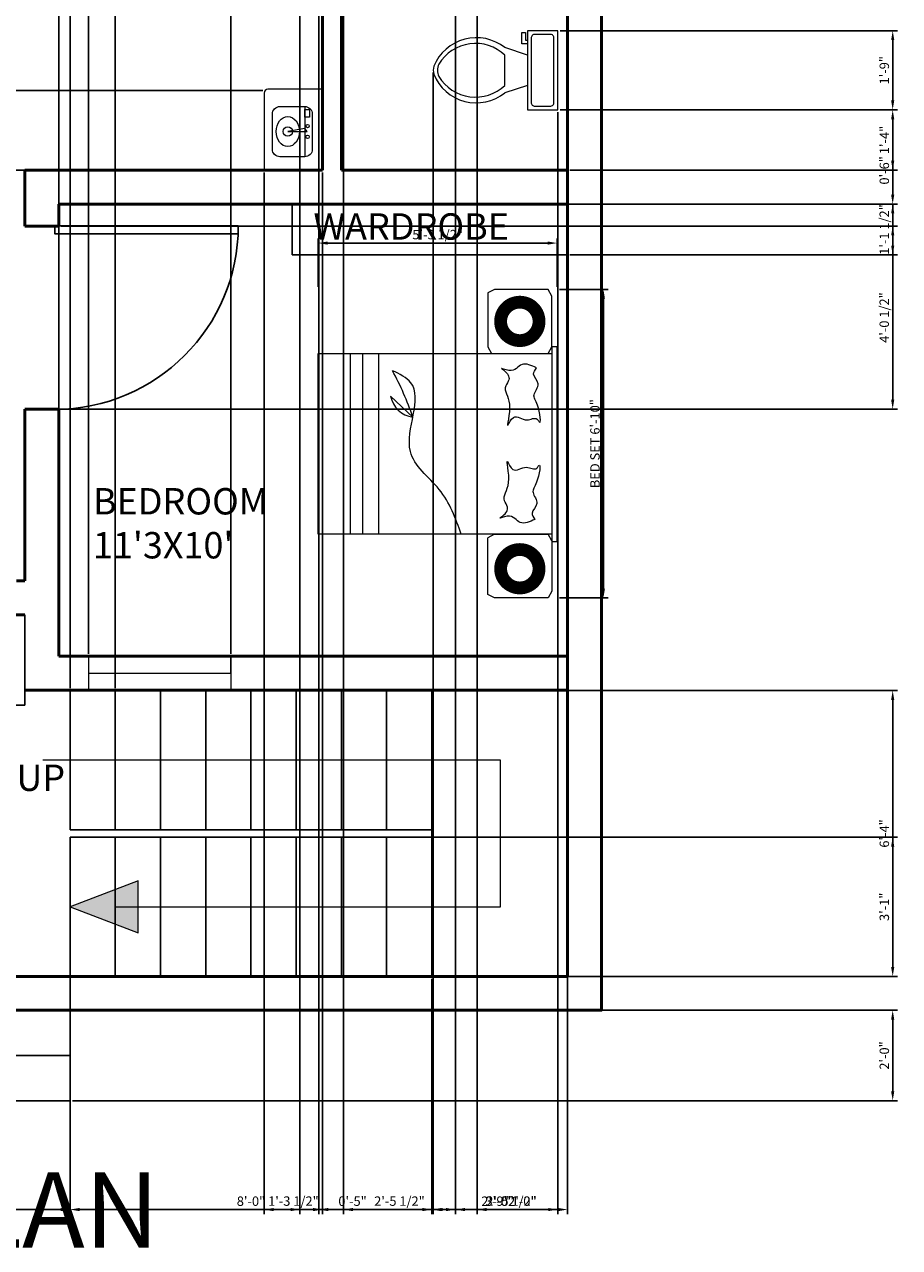
# Model space of a CAD drawing. Units: inches. Extents: x 1854 to 2268, y 1958 to 2535.
# Tile 2 of 4: x 2035 to 2268, y 1958 to 2283. Entities that reach past the tile are written whole.
import ezdxf

# ---------------------------------------------------------------- set-up
doc = ezdxf.new("R2010")
doc.units = ezdxf.units.IN
for name, color, linetype, lineweight in [('A-ANNO-DIMS', 2, 'Continuous', 18), ('A-ANNO-SYMB', 7, 'Continuous', 18), ('A-ANNO-TEXT', 7, 'Continuous', 25), ('A-AREA-IDEN', 7, 'Continuous', 25), ('A-DOOR', 3, 'Continuous', 25), ('A-FLOR-CASE', 30, 'Continuous', 25), ('A-FLOR-FIXT', 9, 'Continuous', 18), ('A-FLOR-STRS', 7, 'Continuous', 25), ('A-FURN', 8, 'Continuous', 18), ('A-GLAZ', 4, 'Continuous', 18), ('A-WALL', 7, 'Continuous', 50)]:
    doc.layers.add(name, color=color, linetype=linetype, lineweight=lineweight)
doc.styles.get("Standard").update_dxf_attribs({"font": 'arial.ttf'})
doc.dimstyles.new('ISO-25', dxfattribs={"dimtxt": 2.5, "dimasz": 2.5, "dimexe": 1.25, "dimexo": 0.625, "dimtad": 1, "dimdec": 0, "dimlunit": 3, "dimtxsty": 'Standard', "dimcen": 2.5, "dimadec": 0, "dimazin": 0, "dimtfac": 1, "dimtdec": 0, "dimtmove": 0, "dimatfit": 3, "dimfxl": 1, "dimarcsym": 0})

# ---------------------------------------------------------------- blocks, each defined once
blk = doc.blocks.new('bed 123')
for p, q in [((-25.76, 31), (25.94, 31)), ((25.94, 32.39), (-25.74, 32.39)), ((-25.74, 32.39), (-25.74, 31)), ((25.76, 31), (24, 30.06)), ((24, 15.76), (24, 30.06)), ((25.76, 31), (39.15, 31)), ((25.94, 31), (25.94, 32.39)), ((39.15, 31), (40.91, 30.06)), ((40.91, 30.06), (40.91, 15.76)), ((24, 15.76), (24.94, 14)), ((39.97, 14), (24.94, 14)), ((40.91, 15.76), (39.97, 14)), ((24, 2.1), (24, -31)), ((-7.1, -5.89), (-12.68, -11.78)), ((-24, -15.04), (24, -15.04)), ((-24, -19.27), (24, -19.27)), ((-24, -22.54), (24, -22.54)), ((-10.17, -31), (-7.61, -31.01))]:
    blk.add_line(p, q)
for points in [[(-25.76, 31), (-39.24, 31), (-41, 30.06), (-41, 15.76), (-40.06, 14), (-25.76, 14), (-24, 14.94), (-24, 30.06)], [(-24, 31), (24, 31), (24, -31), (-24, -31)]]:
    blk.add_lwpolyline(points, close=True)
at = {"const_width": 3.4}
for points in [[(-37.6, 22.5, 1), (-27.4, 22.5, 1)], [(28.06, 22.5, 1), (38.25, 22.5, 1)]]:
    blk.add_lwpolyline(points, format="xyb", close=True, dxfattribs=at)
for centre, radius, start, end in [((18.98, -82.09), 80.54, 108.8924, 118.4699), ((-13.83, -5.1), 6.78, 279.7804, 353.3519)]:
    blk.add_arc(centre, radius, start, end)
for points, knots in [([(-20.15, 26.95), (-19.6, 26.55), (-18.19, 25.51), (-15.93, 28.42), (-12.93, 25.48), (-10.53, 27.62), (-4.31, 28.37), (-7.37, 26.8), (-5.38, 23.99), (-8.44, 20.96), (-2.62, 18.36), (-11.44, 21), (-14.41, 17.7), (-17.27, 20.15), (-18.97, 19.07), (-20.5, 16.88), (-18.47, 20.9), (-22.11, 22.82), (-20.81, 25.56), (-20.15, 26.95)], [0, 0, 0, 0, 1.83091, 4.653214, 7.743318, 10.66504, 15.119925, 15.953636, 18.69724, 22.356007, 24.774329, 30.270914, 35.21341, 37.060797, 39.714351, 40.728626, 42.795822, 46.625816, 50.594847, 50.594847, 50.594847, 50.594847]), ([(20.06, 26.52), (19.49, 26.12), (18.07, 25.12), (15.87, 28.07), (12.81, 25.2), (10.45, 27.4), (4.25, 28.28), (7.28, 26.65), (5.23, 23.88), (8.23, 20.78), (2.35, 18.31), (11.22, 20.76), (14.12, 17.4), (17.03, 19.78), (18.71, 18.67), (20.2, 16.44), (18.25, 20.5), (21.92, 22.34), (20.69, 25.11), (20.06, 26.52)], [0, 0, 0, 0, 1.83091, 4.653214, 7.743318, 10.66504, 15.119925, 15.953636, 18.69724, 22.356007, 24.774329, 30.270914, 35.21341, 37.060797, 39.714351, 40.728626, 42.795822, 46.625816, 50.594847, 50.594847, 50.594847, 50.594847]), ([(24, 6.96), (19.8, 5.46), (11.61, 2.51), (2.01, -11.3), (-14.71, -1.57), (-18.5, -9.41), (-19.41, -11.29)], [0, 0, 0, 0, 13.291621, 25.945947, 44.21489, 49.956985, 49.956985, 49.956985, 49.956985])]:
    blk.add_open_spline(points, degree=3, knots=knots)
blk = doc.blocks.new('*U10')
for p, q in [((9.5, -6), (9.5, -2)), ((-10, -8.5), (-8, -8.5)), ((-10, -9.5), (-10, -8.5)), ((-7, -9.5), (-10, -9.5)), ((-8, -8.5), (-8, -8)), ((-7, -8), (-7, -9.5)), ((-4, -8), (-6, -14)), ((4, -8), (6, -14)), ((4, -14), (-4, -14))]:
    blk.add_line(p, q)
blk.add_lwpolyline([(10.5, -8), (10.5, 0), (-10.5, 0), (-10.5, -8)], close=True)
for points in [[(-9.5, -2), (-9.5, -6)], [(8.5, -1), (-8.5, -1)], [(-8.5, -7), (8.5, -7)]]:
    blk.add_lwpolyline(points)
for centre, radius, start, end in [((-8.62, -1.88), 0.884, 81.8699, 188.1301), ((8.62, -1.88), 0.884, 351.8699, 98.1301), ((-8.62, -6.12), 0.884, 171.8699, 278.1301), ((8.62, -6.12), 0.884, 261.8699, 8.1301), ((3.52, -21.58), 12.17, 141.4691, 247.9714), ((4.2, -21.82), 11.33, 136.3677, 238.9468), ((-3.52, -21.58), 12.17, 292.0284, 38.5307), ((-4.2, -21.82), 11.33, 301.053, 43.6321), ((0, -27.88), 4, 245.7318, 294.2682), ((0, -29), 4, 254.8605, 285.1395)]:
    blk.add_arc(centre, radius, start, end)
blk = doc.blocks.new('*U13')
for p, q in [((-40, 0), (-40, 6)), ((0, 0), (0, 6))]:
    blk.add_line(p, q)
blk.add_lwpolyline([(0, 0), (0, -40), (-1.75, -40), (-1.75, 0)], close=True)
blk.add_arc((0, 0), 40, 180, 270)
blk = doc.blocks.new('*D23')
at = {"layer": 'A-ANNO-DIMS', "color": 0, "lineweight": -2, "transparency": 16777216}
for p, q in [((2177.29, 2212.2), (2190.2, 2212.2)), ((2188.95, 2209.7), (2188.95, 2132.79)), ((2177.29, 2130.29), (2190.2, 2130.29))]:
    blk.add_line(p, q, dxfattribs=at)
at = {"layer": 'A-ANNO-DIMS', "color": 0, "transparency": 16777216}
for points in [[(2188.53, 2209.7), (2189.36, 2209.7), (2188.95, 2212.2)], [(2188.53, 2132.79), (2189.36, 2132.79), (2188.95, 2130.29)]]:
    blk.add_solid(points, dxfattribs=at)
at = {"layer": 'Defpoints', "color": 0, "transparency": 16777216}
for p in [(2176.66, 2212.2), (2176.66, 2130.29), (2188.95, 2130.29)]:
    blk.add_point(p, dxfattribs=at)
at = {"layer": 'A-ANNO-DIMS', "color": 0, "transparency": 16777216, "insert": (2187.03, 2171.25), "char_height": 2.5, "attachment_point": 5, "rotation": 90}
blk.add_mtext('BED SET 6\'-10"', dxfattribs=at)
blk = doc.blocks.new('*D24')
at = {"layer": 'A-ANNO-DIMS', "color": 0, "lineweight": -2, "transparency": 16777216}
for p, q in [((2113.26, 2212.83), (2113.26, 2225.74)), ((2115.76, 2224.49), (2174.16, 2224.49)), ((2176.66, 2212.83), (2176.66, 2225.74))]:
    blk.add_line(p, q, dxfattribs=at)
at = {"layer": 'A-ANNO-DIMS', "color": 0, "transparency": 16777216}
for points in [[(2115.76, 2224.91), (2115.76, 2224.07), (2113.26, 2224.49)], [(2174.16, 2224.91), (2174.16, 2224.07), (2176.66, 2224.49)]]:
    blk.add_solid(points, dxfattribs=at)
at = {"layer": 'Defpoints', "color": 0, "transparency": 16777216}
for p in [(2176.66, 2224.49), (2113.26, 2212.2), (2176.66, 2212.2)]:
    blk.add_point(p, dxfattribs=at)
at = {"layer": 'A-ANNO-DIMS', "color": 0, "transparency": 16777216, "insert": (2144.96, 2226.41), "char_height": 2.5, "attachment_point": 5}
blk.add_mtext('5\'-3 1/2"', dxfattribs=at)
blk = doc.blocks.new('*D36')
at = {"layer": 'A-ANNO-DIMS', "color": 0, "lineweight": -2, "transparency": 16777216}
for p, q in [((2119.96, 2378.21), (2119.96, 1966.69)), ((2149.7, 2378.21), (2149.7, 1966.69)), ((2122.46, 1967.94), (2147.2, 1967.94))]:
    blk.add_line(p, q, dxfattribs=at)
at = {"layer": 'A-ANNO-DIMS', "color": 0, "transparency": 16777216}
for points in [[(2122.46, 1968.36), (2122.46, 1967.52), (2119.96, 1967.94)], [(2147.2, 1968.36), (2147.2, 1967.52), (2149.7, 1967.94)]]:
    blk.add_solid(points, dxfattribs=at)
at = {"layer": 'Defpoints', "color": 0, "transparency": 16777216}
for p in [(2119.96, 2378.84), (2149.7, 2378.84), (2149.7, 1967.94)]:
    blk.add_point(p, dxfattribs=at)
at = {"layer": 'A-ANNO-DIMS', "color": 0, "transparency": 16777216, "insert": (2134.83, 1969.86), "char_height": 2.5, "attachment_point": 5}
blk.add_mtext('2\'-5 1/2"', dxfattribs=at)
blk = doc.blocks.new('*D38')
at = {"layer": 'A-ANNO-DIMS', "color": 0, "lineweight": -2, "transparency": 16777216}
for p, q in [((2045.06, 2229.02), (2266.96, 2229.02)), ((2265.71, 2226.52), (2265.71, 2182.92)), ((2045.06, 2180.42), (2266.96, 2180.42))]:
    blk.add_line(p, q, dxfattribs=at)
at = {"layer": 'A-ANNO-DIMS', "color": 0, "transparency": 16777216}
for points in [[(2265.29, 2226.52), (2266.13, 2226.52), (2265.71, 2229.02)], [(2265.29, 2182.92), (2266.13, 2182.92), (2265.71, 2180.42)]]:
    blk.add_solid(points, dxfattribs=at)
at = {"layer": 'Defpoints', "color": 0, "transparency": 16777216}
for p in [(2044.43, 2229.02), (2044.43, 2180.42), (2265.71, 2180.42)]:
    blk.add_point(p, dxfattribs=at)
at = {"layer": 'A-ANNO-DIMS', "color": 0, "transparency": 16777216, "insert": (2263.79, 2204.72), "char_height": 2.5, "attachment_point": 5, "rotation": 90}
blk.add_mtext('4\'-0 1/2"', dxfattribs=at)
blk = doc.blocks.new('*D43')
at = {"layer": 'A-ANNO-DIMS', "color": 0, "lineweight": -2, "transparency": 16777216}
for p, q in [((2052.36, 2115.46), (2052.36, 2530.99)), ((2054.86, 2529.74), (2087.6, 2529.74)), ((2090.1, 2115.46), (2090.1, 2530.99))]:
    blk.add_line(p, q, dxfattribs=at)
at = {"layer": 'A-ANNO-DIMS', "color": 0, "transparency": 16777216}
for points in [[(2054.86, 2530.16), (2054.86, 2529.32), (2052.36, 2529.74)], [(2087.6, 2530.16), (2087.6, 2529.32), (2090.1, 2529.74)]]:
    blk.add_solid(points, dxfattribs=at)
at = {"layer": 'Defpoints', "color": 0, "transparency": 16777216}
for p in [(2090.1, 2529.74), (2052.36, 2114.84), (2090.1, 2114.84)]:
    blk.add_point(p, dxfattribs=at)
at = {"layer": 'A-ANNO-DIMS', "color": 0, "transparency": 16777216, "insert": (2071.23, 2531.66), "char_height": 2.5, "attachment_point": 5}
blk.add_mtext('3\'-1 1/2"', dxfattribs=at)
blk = doc.blocks.new('*D45')
at = {"layer": 'A-ANNO-DIMS', "color": 0, "lineweight": -2, "transparency": 16777216}
for p, q in [((1906.99, 2001.07), (1906.99, 1966.69)), ((2047.43, 1996.21), (2047.43, 1966.69)), ((1909.49, 1967.94), (2044.93, 1967.94))]:
    blk.add_line(p, q, dxfattribs=at)
at = {"layer": 'A-ANNO-DIMS', "color": 0, "transparency": 16777216}
for points in [[(1909.49, 1968.36), (1909.49, 1967.52), (1906.99, 1967.94)], [(2044.93, 1968.36), (2044.93, 1967.52), (2047.43, 1967.94)]]:
    blk.add_solid(points, dxfattribs=at)
at = {"layer": 'Defpoints', "color": 0, "transparency": 16777216}
for p in [(1906.99, 2001.7), (2047.43, 1996.84), (2047.43, 1967.94)]:
    blk.add_point(p, dxfattribs=at)
at = {"layer": 'A-ANNO-DIMS', "color": 0, "transparency": 16777216, "insert": (1977.21, 1969.86), "char_height": 2.5, "attachment_point": 5}
blk.add_mtext('11\'-8 1/2"', dxfattribs=at)
blk = doc.blocks.new('*D46')
at = {"layer": 'A-ANNO-DIMS', "color": 0, "lineweight": -2, "transparency": 16777216}
for p, q in [((2048.06, 2020.84), (2266.96, 2020.84)), ((2265.71, 2018.34), (2265.71, 1999.34)), ((2048.06, 1996.84), (2266.96, 1996.84))]:
    blk.add_line(p, q, dxfattribs=at)
at = {"layer": 'A-ANNO-DIMS', "color": 0, "transparency": 16777216}
for points in [[(2265.29, 2018.34), (2266.13, 2018.34), (2265.71, 2020.84)], [(2265.29, 1999.34), (2266.13, 1999.34), (2265.71, 1996.84)]]:
    blk.add_solid(points, dxfattribs=at)
at = {"layer": 'Defpoints', "color": 0, "transparency": 16777216}
for p in [(2047.43, 2020.84), (2047.43, 1996.84), (2265.71, 1996.84)]:
    blk.add_point(p, dxfattribs=at)
at = {"layer": 'A-ANNO-DIMS', "color": 0, "transparency": 16777216, "insert": (2263.81, 2008.84), "char_height": 2.5, "attachment_point": 5, "rotation": 90}
blk.add_mtext('2\'-0"', dxfattribs=at)
blk = doc.blocks.new('*D47')
at = {"layer": 'A-ANNO-DIMS', "color": 0, "lineweight": -2, "transparency": 16777216}
for p, q in [((2143.43, 2029.22), (2143.43, 1966.69)), ((2047.43, 2020.21), (2047.43, 1966.69)), ((2049.93, 1967.94), (2140.93, 1967.94))]:
    blk.add_line(p, q, dxfattribs=at)
at = {"layer": 'A-ANNO-DIMS', "color": 0, "transparency": 16777216}
for points in [[(2049.93, 1968.36), (2049.93, 1967.52), (2047.43, 1967.94)], [(2140.93, 1968.36), (2140.93, 1967.52), (2143.43, 1967.94)]]:
    blk.add_solid(points, dxfattribs=at)
at = {"layer": 'Defpoints', "color": 0, "transparency": 16777216}
for p in [(2143.43, 2029.84), (2047.43, 2020.84), (2143.43, 1967.94)]:
    blk.add_point(p, dxfattribs=at)
at = {"layer": 'A-ANNO-DIMS', "color": 0, "transparency": 16777216, "insert": (2095.43, 1969.84), "char_height": 2.5, "attachment_point": 5}
blk.add_mtext('8\'-0"', dxfattribs=at)
blk = doc.blocks.new('*D48')
at = {"layer": 'A-ANNO-DIMS', "color": 0, "lineweight": -2, "transparency": 16777216}
for p, q in [((2144.06, 2105.7), (2266.96, 2105.7)), ((2265.71, 2032.34), (2265.71, 2103.2)), ((2144.06, 2029.84), (2266.96, 2029.84))]:
    blk.add_line(p, q, dxfattribs=at)
at = {"layer": 'A-ANNO-DIMS', "color": 0, "transparency": 16777216}
for points in [[(2265.29, 2103.2), (2266.13, 2103.2), (2265.71, 2105.7)], [(2265.29, 2032.34), (2266.13, 2032.34), (2265.71, 2029.84)]]:
    blk.add_solid(points, dxfattribs=at)
at = {"layer": 'Defpoints', "color": 0, "transparency": 16777216}
for p in [(2143.43, 2105.7), (2265.71, 2105.7), (2143.43, 2029.84)]:
    blk.add_point(p, dxfattribs=at)
at = {"layer": 'A-ANNO-DIMS', "color": 0, "transparency": 16777216, "insert": (2263.81, 2067.77), "char_height": 2.5, "attachment_point": 5, "rotation": 90}
blk.add_mtext('6\'-4"', dxfattribs=at)
blk = doc.blocks.new('*D52')
at = {"layer": 'A-ANNO-DIMS', "color": 0, "lineweight": -2, "transparency": 16777216}
for p, q in [((2149.7, 2378.21), (2149.7, 1966.69)), ((2179.43, 2378.21), (2179.43, 1966.69)), ((2152.2, 1967.94), (2176.93, 1967.94))]:
    blk.add_line(p, q, dxfattribs=at)
at = {"layer": 'A-ANNO-DIMS', "color": 0, "transparency": 16777216}
for points in [[(2152.2, 1968.36), (2152.2, 1967.52), (2149.7, 1967.94)], [(2176.93, 1968.36), (2176.93, 1967.52), (2179.43, 1967.94)]]:
    blk.add_solid(points, dxfattribs=at)
at = {"layer": 'Defpoints', "color": 0, "transparency": 16777216}
for p in [(2149.7, 2378.84), (2179.43, 2378.84), (2179.43, 1967.94)]:
    blk.add_point(p, dxfattribs=at)
at = {"layer": 'A-ANNO-DIMS', "color": 0, "transparency": 16777216, "insert": (2164.57, 1969.86), "char_height": 2.5, "attachment_point": 5}
blk.add_mtext('2\'-5 1/2"', dxfattribs=at)
blk = doc.blocks.new('*D56')
at = {"layer": 'A-ANNO-DIMS', "color": 0, "lineweight": -2, "transparency": 16777216}
for p, q in [((2155.43, 2410.58), (2155.43, 1966.69)), ((2179.43, 2410.58), (2179.43, 1966.69)), ((2157.93, 1967.94), (2176.93, 1967.94))]:
    blk.add_line(p, q, dxfattribs=at)
at = {"layer": 'A-ANNO-DIMS', "color": 0, "transparency": 16777216}
for points in [[(2157.93, 1968.36), (2157.93, 1967.52), (2155.43, 1967.94)], [(2176.93, 1968.36), (2176.93, 1967.52), (2179.43, 1967.94)]]:
    blk.add_solid(points, dxfattribs=at)
at = {"layer": 'Defpoints', "color": 0, "transparency": 16777216}
for p in [(2155.43, 2411.2), (2179.43, 2411.2), (2179.43, 1967.94)]:
    blk.add_point(p, dxfattribs=at)
at = {"layer": 'A-ANNO-DIMS', "color": 0, "transparency": 16777216, "insert": (2167.43, 1969.84), "char_height": 2.5, "attachment_point": 5}
blk.add_mtext('2\'-0"', dxfattribs=at)
blk = doc.blocks.new('*D58')
at = {"layer": 'A-ANNO-DIMS', "color": 0, "lineweight": -2, "transparency": 16777216}
for p, q in [((2098.94, 2243.21), (2098.94, 1966.69)), ((2114.43, 2243.21), (2114.43, 1966.69)), ((2111.93, 1967.94), (2101.44, 1967.94))]:
    blk.add_line(p, q, dxfattribs=at)
at = {"layer": 'A-ANNO-DIMS', "color": 0, "transparency": 16777216}
for points in [[(2101.44, 1968.36), (2101.44, 1967.52), (2098.94, 1967.94)], [(2111.93, 1968.36), (2111.93, 1967.52), (2114.43, 1967.94)]]:
    blk.add_solid(points, dxfattribs=at)
at = {"layer": 'Defpoints', "color": 0, "transparency": 16777216}
for p in [(2098.94, 2243.84), (2114.43, 2243.84), (2098.94, 1967.94)]:
    blk.add_point(p, dxfattribs=at)
at = {"layer": 'A-ANNO-DIMS', "color": 0, "transparency": 16777216, "insert": (2106.69, 1969.86), "char_height": 2.5, "attachment_point": 5}
blk.add_mtext('1\'-3 1/2"', dxfattribs=at)
blk = doc.blocks.new('*D59')
at = {"layer": 'A-ANNO-DIMS', "color": 0, "lineweight": -2, "transparency": 16777216}
for p, q in [((2098.61, 2265.03), (1858.28, 2265.03)), ((1859.53, 2246.34), (1859.53, 2262.53)), ((2098.32, 2243.84), (1858.28, 2243.84))]:
    blk.add_line(p, q, dxfattribs=at)
at = {"layer": 'A-ANNO-DIMS', "color": 0, "transparency": 16777216}
for points in [[(1859.12, 2262.53), (1859.95, 2262.53), (1859.53, 2265.03)], [(1859.12, 2246.34), (1859.95, 2246.34), (1859.53, 2243.84)]]:
    blk.add_solid(points, dxfattribs=at)
at = {"layer": 'Defpoints', "color": 0, "transparency": 16777216}
for p in [(1859.53, 2265.03), (2099.24, 2265.03), (2098.94, 2243.84)]:
    blk.add_point(p, dxfattribs=at)
at = {"layer": 'A-ANNO-DIMS', "color": 0, "transparency": 16777216, "insert": (1857.63, 2254.43), "char_height": 2.5, "attachment_point": 5, "rotation": 90}
blk.add_mtext('1\'-9"', dxfattribs=at)
blk = doc.blocks.new('*D60')
at = {"layer": 'A-ANNO-DIMS', "color": 0, "lineweight": -2, "transparency": 16777216}
for p, q in [((2177.43, 2280.86), (2266.96, 2280.86)), ((2265.71, 2262.36), (2265.71, 2278.36)), ((2177.43, 2259.86), (2266.96, 2259.86))]:
    blk.add_line(p, q, dxfattribs=at)
at = {"layer": 'A-ANNO-DIMS', "color": 0, "transparency": 16777216}
for points in [[(2265.29, 2278.36), (2266.13, 2278.36), (2265.71, 2280.86)], [(2265.29, 2262.36), (2266.13, 2262.36), (2265.71, 2259.86)]]:
    blk.add_solid(points, dxfattribs=at)
at = {"layer": 'Defpoints', "color": 0, "transparency": 16777216}
for p in [(2176.81, 2280.86), (2265.71, 2280.86), (2176.81, 2259.86)]:
    blk.add_point(p, dxfattribs=at)
at = {"layer": 'A-ANNO-DIMS', "color": 0, "transparency": 16777216, "insert": (2263.81, 2270.36), "char_height": 2.5, "attachment_point": 5, "rotation": 90}
blk.add_mtext('1\'-9"', dxfattribs=at)
blk = doc.blocks.new('*D61')
at = {"layer": 'A-ANNO-DIMS', "color": 0, "lineweight": -2, "transparency": 16777216}
for p, q in [((2143.81, 2269.73), (2143.81, 1966.69)), ((2176.81, 2259.23), (2176.81, 1966.69)), ((2146.31, 1967.94), (2174.31, 1967.94))]:
    blk.add_line(p, q, dxfattribs=at)
at = {"layer": 'A-ANNO-DIMS', "color": 0, "transparency": 16777216}
for points in [[(2146.31, 1968.36), (2146.31, 1967.52), (2143.81, 1967.94)], [(2174.31, 1968.36), (2174.31, 1967.52), (2176.81, 1967.94)]]:
    blk.add_solid(points, dxfattribs=at)
at = {"layer": 'Defpoints', "color": 0, "transparency": 16777216}
for p in [(2143.81, 2270.36), (2176.81, 2259.86), (2176.81, 1967.94)]:
    blk.add_point(p, dxfattribs=at)
at = {"layer": 'A-ANNO-DIMS', "color": 0, "transparency": 16777216, "insert": (2160.31, 1969.84), "char_height": 2.5, "attachment_point": 5}
blk.add_mtext('2\'-9"', dxfattribs=at)
blk = doc.blocks.new('*D62')
at = {"layer": 'A-ANNO-DIMS', "color": 0, "lineweight": -2, "transparency": 16777216}
for p, q in [((2177.43, 2259.86), (2266.96, 2259.86)), ((2265.71, 2257.36), (2265.71, 2246.34)), ((2180.06, 2243.84), (2266.96, 2243.84))]:
    blk.add_line(p, q, dxfattribs=at)
at = {"layer": 'A-ANNO-DIMS', "color": 0, "transparency": 16777216}
for points in [[(2265.29, 2257.36), (2266.13, 2257.36), (2265.71, 2259.86)], [(2265.29, 2246.34), (2266.13, 2246.34), (2265.71, 2243.84)]]:
    blk.add_solid(points, dxfattribs=at)
at = {"layer": 'Defpoints', "color": 0, "transparency": 16777216}
for p in [(2176.81, 2259.86), (2179.43, 2243.84), (2265.71, 2243.84)]:
    blk.add_point(p, dxfattribs=at)
at = {"layer": 'A-ANNO-DIMS', "color": 0, "transparency": 16777216, "insert": (2263.83, 2251.85), "char_height": 2.5, "attachment_point": 5, "rotation": 90}
blk.add_mtext('1\'-4"', dxfattribs=at)
blk = doc.blocks.new('*D63')
at = {"layer": 'A-ANNO-DIMS', "color": 0, "lineweight": -2, "transparency": 16777216}
for p, q in [((2143.43, 2029.22), (2143.43, 1966.69)), ((2179.43, 2029.21), (2179.43, 1966.69)), ((2145.93, 1967.94), (2176.93, 1967.94))]:
    blk.add_line(p, q, dxfattribs=at)
at = {"layer": 'A-ANNO-DIMS', "color": 0, "transparency": 16777216}
for points in [[(2145.93, 1968.36), (2145.93, 1967.52), (2143.43, 1967.94)], [(2176.93, 1968.36), (2176.93, 1967.52), (2179.43, 1967.94)]]:
    blk.add_solid(points, dxfattribs=at)
at = {"layer": 'Defpoints', "color": 0, "transparency": 16777216}
for p in [(2143.43, 2029.84), (2179.43, 2029.84), (2179.43, 1967.94)]:
    blk.add_point(p, dxfattribs=at)
at = {"layer": 'A-ANNO-DIMS', "color": 0, "transparency": 16777216, "insert": (2161.43, 1969.84), "char_height": 2.5, "attachment_point": 5}
blk.add_mtext('3\'-0"', dxfattribs=at)
blk = doc.blocks.new('*D64')
at = {"layer": 'A-ANNO-DIMS', "color": 0, "lineweight": -2, "transparency": 16777216}
for p, q in [((2144.06, 2066.77), (2266.96, 2066.77)), ((2265.71, 2032.34), (2265.71, 2064.27)), ((2144.06, 2029.84), (2266.96, 2029.84))]:
    blk.add_line(p, q, dxfattribs=at)
at = {"layer": 'A-ANNO-DIMS', "color": 0, "transparency": 16777216}
for points in [[(2265.29, 2064.27), (2266.13, 2064.27), (2265.71, 2066.77)], [(2265.29, 2032.34), (2266.13, 2032.34), (2265.71, 2029.84)]]:
    blk.add_solid(points, dxfattribs=at)
at = {"layer": 'Defpoints', "color": 0, "transparency": 16777216}
for p in [(2143.43, 2066.77), (2265.71, 2066.77), (2143.43, 2029.84)]:
    blk.add_point(p, dxfattribs=at)
at = {"layer": 'A-ANNO-DIMS', "color": 0, "transparency": 16777216, "insert": (2263.81, 2048.31), "char_height": 2.5, "attachment_point": 5, "rotation": 90}
blk.add_mtext('3\'-1"', dxfattribs=at)
blk = doc.blocks.new('*D65')
at = {"layer": 'A-ANNO-DIMS', "color": 0, "lineweight": -2, "transparency": 16777216}
for p, q in [((2047.43, 2106.33), (2047.43, 2530.99)), ((2049.93, 2529.74), (2056.93, 2529.74)), ((2059.43, 2106.33), (2059.43, 2530.99))]:
    blk.add_line(p, q, dxfattribs=at)
at = {"layer": 'A-ANNO-DIMS', "color": 0, "transparency": 16777216}
for points in [[(2049.93, 2530.16), (2049.93, 2529.32), (2047.43, 2529.74)], [(2056.93, 2530.16), (2056.93, 2529.32), (2059.43, 2529.74)]]:
    blk.add_solid(points, dxfattribs=at)
at = {"layer": 'Defpoints', "color": 0, "transparency": 16777216}
for p in [(2059.43, 2529.74), (2047.43, 2105.7), (2059.43, 2105.7)]:
    blk.add_point(p, dxfattribs=at)
at = {"layer": 'A-ANNO-DIMS', "color": 0, "transparency": 16777216, "insert": (2053.43, 2531.64), "char_height": 2.5, "attachment_point": 5}
blk.add_mtext('1\'-0"', dxfattribs=at)
blk = doc.blocks.new('*D66')
at = {"layer": 'A-ANNO-DIMS', "color": 0, "lineweight": -2, "transparency": 16777216}
for p, q in [((2044.43, 2115.46), (2044.43, 2530.99)), ((2046.93, 2529.74), (2049.86, 2529.74)), ((2052.36, 2115.46), (2052.36, 2530.99))]:
    blk.add_line(p, q, dxfattribs=at)
at = {"layer": 'A-ANNO-DIMS', "color": 0, "transparency": 16777216}
for points in [[(2046.93, 2530.16), (2046.93, 2529.32), (2044.43, 2529.74)], [(2049.86, 2530.16), (2049.86, 2529.32), (2052.36, 2529.74)]]:
    blk.add_solid(points, dxfattribs=at)
at = {"layer": 'Defpoints', "color": 0, "transparency": 16777216}
for p in [(2052.36, 2529.74), (2044.43, 2114.84), (2052.36, 2114.84)]:
    blk.add_point(p, dxfattribs=at)
at = {"layer": 'A-ANNO-DIMS', "color": 0, "transparency": 16777216, "insert": (2048.4, 2531.64), "char_height": 2.5, "attachment_point": 5}
blk.add_mtext('0\'-8"', dxfattribs=at)
blk = doc.blocks.new('*D69')
at = {"layer": 'A-ANNO-DIMS', "color": 0, "lineweight": -2, "transparency": 16777216}
for p, q in [((2265.71, 2237.34), (2265.71, 2247.74)), ((2045.06, 2234.84), (2266.96, 2234.84)), ((2265.71, 2229.02), (2265.71, 2234.84)), ((2045.06, 2229.02), (2266.96, 2229.02)), ((2265.71, 2226.52), (2265.71, 2224.02))]:
    blk.add_line(p, q, dxfattribs=at)
at = {"layer": 'A-ANNO-DIMS', "color": 0, "transparency": 16777216}
for points in [[(2265.29, 2237.34), (2266.13, 2237.34), (2265.71, 2234.84)], [(2265.29, 2226.52), (2266.13, 2226.52), (2265.71, 2229.02)]]:
    blk.add_solid(points, dxfattribs=at)
at = {"layer": 'Defpoints', "color": 0, "transparency": 16777216}
for p in [(2044.43, 2234.84), (2265.71, 2234.84), (2044.43, 2229.02)]:
    blk.add_point(p, dxfattribs=at)
at = {"layer": 'A-ANNO-DIMS', "color": 0, "transparency": 16777216, "insert": (2263.81, 2243.79), "char_height": 2.5, "attachment_point": 5, "rotation": 90}
blk.add_mtext('0\'-6"', dxfattribs=at)
blk = doc.blocks.new('*D77')
at = {"layer": 'A-ANNO-DIMS', "color": 0, "lineweight": -2, "transparency": 16777216}
for p, q in [((2180.06, 2234.84), (2266.96, 2234.84)), ((2265.71, 2232.34), (2265.71, 2223.83)), ((2180.06, 2221.33), (2266.96, 2221.33))]:
    blk.add_line(p, q, dxfattribs=at)
at = {"layer": 'A-ANNO-DIMS', "color": 0, "transparency": 16777216}
for points in [[(2265.29, 2232.34), (2266.13, 2232.34), (2265.71, 2234.84)], [(2265.29, 2223.83), (2266.13, 2223.83), (2265.71, 2221.33)]]:
    blk.add_solid(points, dxfattribs=at)
at = {"layer": 'Defpoints', "color": 0, "transparency": 16777216}
for p in [(2179.43, 2234.84), (2179.43, 2221.33), (2265.71, 2221.33)]:
    blk.add_point(p, dxfattribs=at)
at = {"layer": 'A-ANNO-DIMS', "color": 0, "transparency": 16777216, "insert": (2263.79, 2228.09), "char_height": 2.5, "attachment_point": 5, "rotation": 90}
blk.add_mtext('1\'-1 1/2"', dxfattribs=at)
blk = doc.blocks.new('*D79')
at = {"layer": 'A-ANNO-DIMS', "color": 0, "lineweight": -2, "transparency": 16777216}
for p, q in [((2113.43, 2336.21), (2113.43, 1966.69)), ((2108.43, 2327.21), (2108.43, 1966.69)), ((2105.93, 1967.94), (2103.43, 1967.94)), ((2108.43, 1967.94), (2113.43, 1967.94)), ((2115.93, 1967.94), (2126.33, 1967.94))]:
    blk.add_line(p, q, dxfattribs=at)
at = {"layer": 'A-ANNO-DIMS', "color": 0, "transparency": 16777216}
for points in [[(2105.93, 1968.36), (2105.93, 1967.52), (2108.43, 1967.94)], [(2115.93, 1968.36), (2115.93, 1967.52), (2113.43, 1967.94)]]:
    blk.add_solid(points, dxfattribs=at)
at = {"layer": 'Defpoints', "color": 0, "transparency": 16777216}
for p in [(2113.43, 2336.84), (2108.43, 2327.84), (2113.43, 1967.94)]:
    blk.add_point(p, dxfattribs=at)
at = {"layer": 'A-ANNO-DIMS', "color": 0, "transparency": 16777216, "insert": (2122.38, 1969.84), "char_height": 2.5, "attachment_point": 5}
blk.add_mtext('0\'-5"', dxfattribs=at)

msp = doc.modelspace()

# ---------------------------------------------------------------- hatches: boundary and pattern name
at = {"layer": 'A-ANNO-SYMB'}
h = msp.add_hatch(color=256, dxfattribs=at)
h.set_gradient(color1=(255, 255, 255), tint=1)
h.paths.add_polyline_path([(2059.43, 2052.89), (2047.49, 2048.31), (2059.43, 2043.73)])
h.paths.add_polyline_path([(2065.47, 2055.2), (2059.43, 2052.89), (2059.43, 2048.31), (2065.47, 2048.31)])
h.paths.add_polyline_path([(2065.47, 2048.31), (2059.43, 2048.31), (2059.43, 2043.73), (2065.47, 2041.41)])

# ---------------------------------------------------------------- linework, layer by layer
for p, q in [((2161.65, 2087.24), (2040.16, 2087.24)), ((2161.65, 2048.31), (2161.65, 2087.24)), ((2059.43, 2048.31), (2161.65, 2048.31))]:
    msp.add_line(p, q, dxfattribs=at)
msp.add_lwpolyline([(2047.49, 2048.31), (2065.47, 2041.41), (2065.47, 2055.2)], close=True, dxfattribs=at)
at = {"layer": 'A-FLOR-CASE'}
for p, q in [((2106.37, 2234.84), (2106.37, 2221.33)), ((2106.37, 2221.33), (2179.43, 2221.33))]:
    msp.add_line(p, q, dxfattribs=at)
at = {"layer": 'A-FLOR-FIXT'}
for p, q in [((2098.94, 2264.32), (2098.94, 2243.84)), ((2114.43, 2265.32), (2099.94, 2265.32)), ((2109.7, 2260.74), (2109.7, 2247.4)), ((2109.7, 2254.88), (2105.2, 2254.1)), ((2105.2, 2254.1), (2110.32, 2254.1)), ((2110.32, 2254.1), (2109.7, 2254.88))]:
    msp.add_line(p, q, dxfattribs=at)
msp.add_lwpolyline([(2103.12, 2260.74), (2109.7, 2260.74, -0.414214), (2111.7, 2258.74), (2111.7, 2249.4, -0.414214), (2109.7, 2247.4), (2103.12, 2247.4, -0.414214), (2101.12, 2249.4), (2101.12, 2258.74, -0.414214)], format="xyb", close=True, dxfattribs=at)
msp.add_lwpolyline([(2109.7, 2259.96), (2110.98, 2259.96), (2110.98, 2257.87), (2109.7, 2257.87)], close=True, dxfattribs=at)
for centre, radius in [((2105.2, 2254.1), 1.27), ((2110.46, 2255.55), 0.446), ((2110.46, 2252.69), 0.446)]:
    msp.add_circle(centre, radius, dxfattribs=at)
msp.add_arc((2099.94, 2264.32), 1, 90, 180, dxfattribs=at)
msp.add_ellipse((2105.2, 2254.1), major_axis=(0, -3.99), ratio=0.776702, start_param=-1.570796, end_param=4.712389, dxfattribs=at)
at = {"layer": 'A-FLOR-STRS'}
for p, q in [((2035.43, 2101.79), (2035.43, 2125.84)), ((2047.43, 2068.77), (2047.43, 2105.7)), ((2059.43, 2068.77), (2059.43, 2105.7)), ((2071.43, 2068.77), (2071.43, 2105.7)), ((2083.43, 2068.77), (2083.43, 2105.7)), ((2095.43, 2068.77), (2095.43, 2105.7)), ((2107.43, 2068.77), (2107.43, 2105.7)), ((2119.43, 2068.77), (2119.43, 2105.7)), ((2131.43, 2068.77), (2131.43, 2105.7)), ((2143.43, 2068.77), (2143.43, 2105.7)), ((2179.43, 2029.84), (2179.43, 2105.7)), ((1972.6, 2101.79), (2035.43, 2101.79)), ((2047.43, 2068.77), (2143.43, 2068.77)), ((2143.43, 2029.84), (2143.43, 2068.77)), ((2047.43, 2020.84), (2047.43, 2066.77)), ((2047.43, 2066.77), (2143.43, 2066.77)), ((2059.43, 2029.84), (2059.43, 2066.77)), ((2071.43, 2029.84), (2071.43, 2066.77)), ((2083.43, 2029.84), (2083.43, 2066.77)), ((2095.43, 2029.84), (2095.43, 2066.77)), ((2107.43, 2029.84), (2107.43, 2066.77)), ((2119.43, 2029.84), (2119.43, 2066.77)), ((2131.43, 2029.84), (2131.43, 2066.77)), ((2012.17, 2020.84), (2047.43, 2020.84)), ((2047.43, 2020.84), (2047.43, 1996.84)), ((2012.17, 2008.84), (2047.43, 2008.84)), ((2012.17, 1996.84), (2047.43, 1996.84))]:
    msp.add_line(p, q, dxfattribs=at)
at = {"layer": 'A-GLAZ'}
for p, q in [((2052.36, 2114.84), (2052.36, 2105.84)), ((2090.1, 2110.34), (2090.1, 2114.84)), ((2090.1, 2114.84), (2090.1, 2105.84)), ((2052.36, 2110.34), (2090.1, 2110.34))]:
    msp.add_line(p, q, dxfattribs=at)
at = {"layer": 'A-WALL'}
for p, q in [((2179.43, 2491.84), (2179.43, 2029.84)), ((2114.43, 2290.77), (2114.43, 2243.84)), ((2119.43, 2290.77), (2119.43, 2243.84)), ((2035.43, 2243.84), (2114.43, 2243.84)), ((2035.43, 2229.02), (2035.43, 2243.84)), ((2119.43, 2243.84), (2179.43, 2243.84)), ((2044.43, 2234.84), (2179.43, 2234.84)), ((2044.43, 2229.02), (2044.43, 2234.84)), ((2035.43, 2229.02), (2044.43, 2229.02)), ((2039.93, 2180.42), (2035.43, 2180.42)), ((2035.43, 2180.42), (2044.43, 2180.42)), ((2035.43, 2134.84), (2035.43, 2180.42)), ((2044.43, 2114.84), (2044.43, 2180.42)), ((2033.21, 2134.84), (2035.43, 2134.84)), ((1897.43, 2125.84), (2035.43, 2125.84)), ((2044.43, 2114.84), (2179.43, 2114.84)), ((2035.43, 2105.84), (2179.43, 2105.84)), ((2179.43, 2029.84), (1897.43, 2029.84))]:
    msp.add_line(p, q, dxfattribs=at)
msp.add_lwpolyline([(1888.43, 2500.84), (2188.43, 2500.84), (2188.43, 2020.84), (1888.43, 2020.84)], close=True, dxfattribs=at)

# ---------------------------------------------------------------- block references
at = {"layer": 'A-DOOR', "xscale": 1.216755450299426, "yscale": 1.216755450299426, "zscale": 1.216755450299426, "rotation": 90.00000000000003}
msp.add_blockref('*U13', (2043.39, 2229.04), dxfattribs=at)
at = {"layer": 'A-FLOR-FIXT', "rotation": 270}
msp.add_blockref('*U10', (2176.81, 2270.36), dxfattribs=at)
at = {"layer": 'A-FURN', "rotation": 270}
msp.add_blockref('bed 123', (2144.27, 2171.2), dxfattribs=at)

# ---------------------------------------------------------------- texts
at = {"layer": 'A-ANNO-TEXT', "attachment_point": 1}
for s, insert, char_height in [('WARDROBE', (2112.01, 2232.39), 7), ('UP', (2033.17, 2086.06), 7), ('PLAN', (2002.62, 1977.86), 20)]:
    msp.add_mtext_dynamic_manual_height_columns(s, width=76.0498, gutter_width=12.5, heights=[0], dxfattribs=dict(at, insert=insert, char_height=char_height))
at = {"layer": 'A-AREA-IDEN', "insert": (2053.49, 2159.45), "char_height": 7, "attachment_point": 1}
msp.add_mtext_dynamic_manual_height_columns("BEDROOM\\P11'3X10'", width=76.0498, gutter_width=12.5, heights=[0], dxfattribs=at)

# ---------------------------------------------------------------- dimensions: what is measured, and where the dimension line sits
at = {"layer": 'A-ANNO-DIMS'}
for base, p1, p2, picture, middle in [((2052.36, 2529.74), (2044.43, 2114.84), (2052.36, 2114.84), '*D66', (2048.4, 2531.64)), ((2059.43, 2529.74), (2047.43, 2105.7), (2059.43, 2105.7), '*D65', (2053.43, 2531.64)), ((2090.1, 2529.74), (2052.36, 2114.84), (2090.1, 2114.84), '*D43', (2071.23, 2531.66)), ((2179.43, 1967.94), (2155.43, 2411.2), (2179.43, 2411.2), '*D56', (2167.43, 1969.84)), ((2149.7, 1967.94), (2119.96, 2378.84), (2149.7, 2378.84), '*D36', (2134.83, 1969.86)), ((2179.43, 1967.94), (2149.7, 2378.84), (2179.43, 2378.84), '*D52', (2164.57, 1969.86)), ((2113.43, 1967.94), (2108.43, 2327.84), (2113.43, 2336.84), '*D79', (2122.38, 1969.84)), ((2176.81, 1967.94), (2143.81, 2270.36), (2176.81, 2259.86), '*D61', (2160.31, 1969.84)), ((2098.94, 1967.94), (2114.43, 2243.84), (2098.94, 2243.84), '*D58', (2106.69, 1969.86)), ((2176.66, 2224.49), (2113.26, 2212.2), (2176.66, 2212.2), '*D24', (2144.96, 2226.41)), ((2143.43, 1967.94), (2047.43, 2020.84), (2143.43, 2029.84), '*D47', (2095.43, 1969.84)), ((2179.43, 1967.94), (2143.43, 2029.84), (2179.43, 2029.84), '*D63', (2161.43, 1969.84)), ((2047.43, 1967.94), (1906.99, 2001.7), (2047.43, 1996.84), '*D45', (1977.21, 1969.86))]:
    dim = msp.add_linear_dim(base=base, p1=p1, p2=p2, dimstyle='ISO-25', override={"dimdec": 1, "dimlfac": 1, "dimrnd": 0, "dimzin": 1, "dimdsep": 46, "dimlunit": 4, "dimfrac": 2}, dxfattribs=at)
    dim.commit()
    dim.dimension.update_dxf_attribs({"geometry": picture, "text_midpoint": middle})
for base, p1, p2, picture, middle in [((2265.71, 2280.86), (2176.81, 2259.86), (2176.81, 2280.86), '*D60', (2263.81, 2270.36)), ((1859.53, 2265.03), (2098.94, 2243.84), (2099.24, 2265.03), '*D59', (1857.63, 2254.43)), ((2265.71, 2243.84), (2176.81, 2259.86), (2179.43, 2243.84), '*D62', (2263.83, 2251.85)), ((2265.71, 2234.84), (2044.43, 2229.02), (2044.43, 2234.84), '*D69', (2263.81, 2243.79)), ((2265.71, 2221.33), (2179.43, 2234.84), (2179.43, 2221.33), '*D77', (2263.79, 2228.09)), ((2265.71, 2180.42), (2044.43, 2229.02), (2044.43, 2180.42), '*D38', (2263.79, 2204.72)), ((2265.71, 2105.7), (2143.43, 2029.84), (2143.43, 2105.7), '*D48', (2263.81, 2067.77)), ((2265.71, 2066.77), (2143.43, 2029.84), (2143.43, 2066.77), '*D64', (2263.81, 2048.31)), ((2265.71, 1996.84), (2047.43, 2020.84), (2047.43, 1996.84), '*D46', (2263.81, 2008.84))]:
    dim = msp.add_linear_dim(base=base, p1=p1, p2=p2, angle=90, dimstyle='ISO-25', override={"dimdec": 1, "dimlfac": 1, "dimrnd": 0, "dimzin": 1, "dimdsep": 46, "dimlunit": 4, "dimfrac": 2}, dxfattribs=at)
    dim.commit()
    dim.dimension.update_dxf_attribs({"geometry": picture, "text_midpoint": middle})
dim = msp.add_linear_dim(base=(2188.95, 2130.29), p1=(2176.66, 2212.2), p2=(2176.66, 2130.29), angle=270, text='BED SET <>', dimstyle='ISO-25', override={"dimdec": 1, "dimlfac": 1, "dimrnd": 0, "dimzin": 1, "dimdsep": 46, "dimlunit": 4, "dimfrac": 2}, dxfattribs=at)
dim.commit()
dim.dimension.update_dxf_attribs({"geometry": '*D23', "text_midpoint": (2187.03, 2171.25)})

doc.saveas('drawing.dxf')
